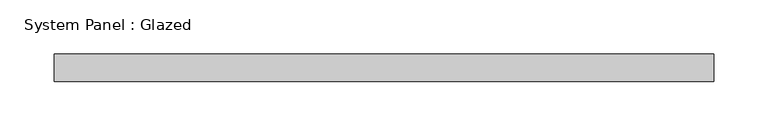
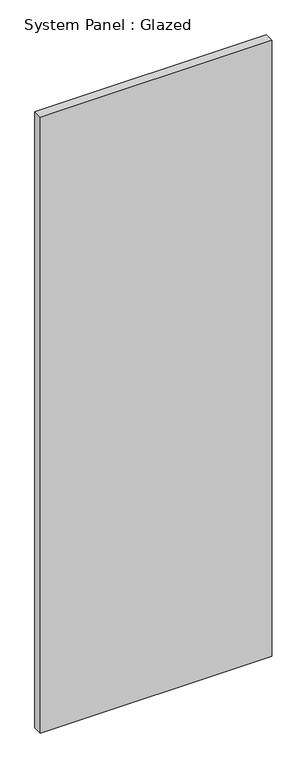
"""IFC4 building model written with IfcOpenShell, lengths in millimetres: plate geometry, System Panel : Glazed."""

from ifc_helpers import new_model, si_unit, origin, origin_with_axes, place, context, project, spatial, polyline, outline, extrude, source, transform, mapped, element, save


def system_panel_glazed_f5cea47f(model_context):
    return source(origin(), model_context, "Body", "SweptSolid", [
        extrude(outline(polyline([(304.8, 19.05), (-304.8, 19.05), (-304.8, 44.45), (304.8, 44.45), (304.8, 19.05)])), origin_with_axes(), (0.0, 0.0, 1.0), 1716.0744962),
    ])


if __name__ == "__main__":
    model = new_model("IFC4")
    model_context = context("Model", 3, world=origin())
    ifc_project = project(units=[si_unit("LENGTHUNIT", "METRE", prefix="MILLI")], contexts=[model_context])
    site = spatial("IfcSite", under=ifc_project)
    building = spatial("IfcBuilding", under=site)
    placement = place(None, origin())
    system_panel_glazed_shape = system_panel_glazed_f5cea47f(model_context)
    element("IfcPlate", 1, ObjectType="System Panel : Glazed", at=placement, inside=building, context=model_context, shape_type="MappedRepresentation", body=[
        mapped(system_panel_glazed_shape, transform((0.0, 0.0, 0.0), x_axis=(1.0, 0.0, 0.0), y_axis=(0.0, 1.0, 0.0), z_axis=(0.0, 0.0, 1.0))),
    ])
    save(model, "model.ifc")

# Revit data of these elements
# Type "System Panel : Glazed"
#   Construction Type Id = "GSP4R"
#   Analytic Construction = "1/8 in Pilkington single glazing"
#   Visual Light Transmittance = 0.9
#   Solar Heat Gain Coefficient = 0.86
#   Heat Transfer Coefficient (U) = 1.18115 BTU/(h·ft²·°F)
#   Define Thermal Properties by = 1
# Element 1 (IfcPlate, "System Panel : Glazed")
#   Materials on its faces: "Glass"
# Materials
#   "Glass": class "Glass", colour RGB 0 128 192, transparency 0.75, Description = "Soda Lime Glass", Cost = 0
